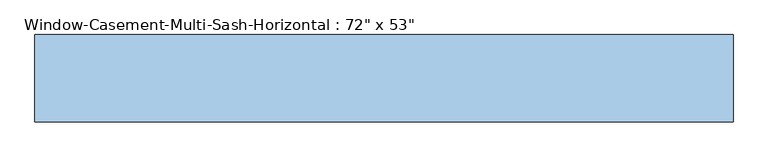
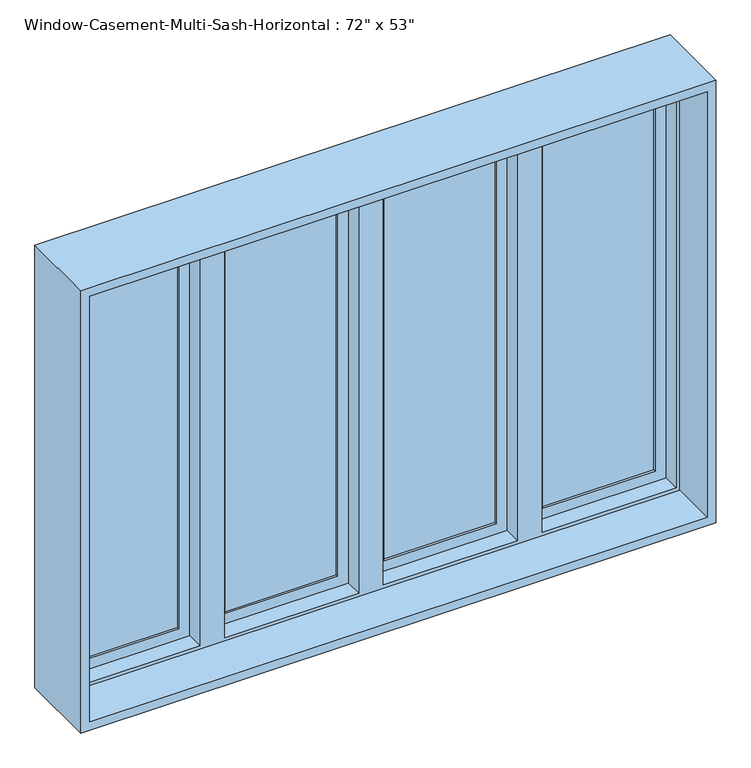
"""IFC4 building model written with IfcOpenShell, lengths in millimetres: window geometry."""

from ifc_helpers import new_model, si_unit, frame, origin, place, context, project, spatial, polyline, outline, extrude, faceted_brep, source, transform, mapped, element, save


def window_5487fb6d(model_context):
    return source(origin(), model_context, "Body", "SolidModel", [
        extrude(outline(polyline([(2235.2, 482.6), (939.8, 482.6), (939.8, 889.0), (2235.2, 889.0), (2235.2, 482.6)]), holes=[polyline([(2193.3296875, 847.1296875), (981.6703125, 847.1296875), (981.6703125, 524.4703125), (2193.3296875, 524.4703125), (2193.3296875, 847.1296875)])]), frame((0.0, 73.025, 0.0), z_axis=(0.0, 1.0, 0.0), x_axis=(0.0, 0.0, 1.0)), (0.0, 0.0, 1.0), 31.75),
        extrude(outline(polyline([(2235.2, -889.0), (939.8, -889.0), (939.8, -482.6), (2235.2, -482.6), (2235.2, -889.0)]), holes=[polyline([(2193.3296875, -524.4703125), (981.6703125, -524.4703125), (981.6703125, -847.1296875), (2193.3296875, -847.1296875), (2193.3296875, -524.4703125)])]), frame((0.0, 73.025, 0.0), z_axis=(0.0, 1.0, 0.0), x_axis=(0.0, 0.0, 1.0)), (0.0, 0.0, 1.0), 31.75),
        extrude(outline(polyline([(-524.4703125, 98.425), (-524.4703125, 92.075), (-847.1296875, 92.075), (-847.1296875, 98.425), (-524.4703125, 98.425)])), frame((0.0, 0.0, 981.6703125), z_axis=(0.0, 0.0, 1.0), x_axis=(1.0, 0.0, 0.0)), (0.0, 0.0, 1.0), 1211.659375),
        extrude(outline(polyline([(-524.4703125, 85.725), (-524.4703125, 79.375), (-847.1296875, 79.375), (-847.1296875, 85.725), (-524.4703125, 85.725)])), frame((0.0, 0.0, 981.6703125), z_axis=(0.0, 0.0, 1.0), x_axis=(1.0, 0.0, 0.0)), (0.0, 0.0, 1.0), 1211.659375),
        extrude(outline(polyline([(847.1296875, 98.425), (847.1296875, 92.075), (524.4703125, 92.075), (524.4703125, 98.425), (847.1296875, 98.425)])), frame((0.0, 0.0, 981.6703125), z_axis=(0.0, 0.0, 1.0), x_axis=(1.0, 0.0, 0.0)), (0.0, 0.0, 1.0), 1211.659375),
        extrude(outline(polyline([(847.1296875, 85.725), (847.1296875, 79.375), (524.4703125, 79.375), (524.4703125, 85.725), (847.1296875, 85.725)])), frame((0.0, 0.0, 981.6703125), z_axis=(0.0, 0.0, 1.0), x_axis=(1.0, 0.0, 0.0)), (0.0, 0.0, 1.0), 1211.659375),
        extrude(outline(polyline([(-67.2703125, 98.425), (-67.2703125, 92.075), (-389.9296875, 92.075), (-389.9296875, 98.425), (-67.2703125, 98.425)])), frame((0.0, 0.0, 981.6703125), z_axis=(0.0, 0.0, 1.0), x_axis=(1.0, 0.0, 0.0)), (0.0, 0.0, 1.0), 1211.659375),
        extrude(outline(polyline([(-67.2703125, 85.725), (-67.2703125, 79.375), (-389.9296875, 79.375), (-389.9296875, 85.725), (-67.2703125, 85.725)])), frame((0.0, 0.0, 981.6703125), z_axis=(0.0, 0.0, 1.0), x_axis=(1.0, 0.0, 0.0)), (0.0, 0.0, 1.0), 1211.659375),
        extrude(outline(polyline([(389.9296875, 98.425), (389.9296875, 92.075), (67.2703125, 92.075), (67.2703125, 98.425), (389.9296875, 98.425)])), frame((0.0, 0.0, 981.6703125), z_axis=(0.0, 0.0, 1.0), x_axis=(1.0, 0.0, 0.0)), (0.0, 0.0, 1.0), 1211.659375),
        extrude(outline(polyline([(389.9296875, 85.725), (389.9296875, 79.375), (67.2703125, 79.375), (67.2703125, 85.725), (389.9296875, 85.725)])), frame((0.0, 0.0, 981.6703125), z_axis=(0.0, 0.0, 1.0), x_axis=(1.0, 0.0, 0.0)), (0.0, 0.0, 1.0), 1211.659375),
        faceted_brep([(-482.6, 73.025, 2235.2), (-889.0, 73.025, 2235.2), (-889.0, 114.3, 2235.2), (889.0, 114.3, 2235.2), (889.0, 73.025, 2235.2), (482.6, 73.025, 2235.2), (482.6, 111.125, 2235.2), (431.8, 111.125, 2235.2), (431.8, 73.025, 2235.2), (25.4, 73.025, 2235.2), (25.4, 111.125, 2235.2), (-25.4, 111.125, 2235.2), (-25.4, 73.025, 2235.2), (-431.8, 73.025, 2235.2), (-431.8, 111.125, 2235.2), (-482.6, 111.125, 2235.2), (-878.8796875, 22.225, 2225.0796875), (-878.8796875, 73.025, 2225.0796875), (-492.7203125, 73.025, 2225.0796875), (-492.7203125, 22.225, 2225.0796875), (878.8796875, 73.025, 2225.0796875), (878.8796875, 22.225, 2225.0796875), (492.7203125, 22.225, 2225.0796875), (492.7203125, 73.025, 2225.0796875), (-421.6796875, 73.025, 2225.0796875), (-35.5203125, 73.025, 2225.0796875), (-35.5203125, 22.225, 2225.0796875), (-421.6796875, 22.225, 2225.0796875), (35.5203125, 73.025, 2225.0796875), (421.6796875, 73.025, 2225.0796875), (421.6796875, 22.225, 2225.0796875), (35.5203125, 22.225, 2225.0796875), (-889.0, -114.3, 2235.2), (-889.0, 22.225, 2235.2), (889.0, 22.225, 2235.2), (889.0, -114.3, 2235.2), (-914.4, 114.3, 2260.6), (-914.4, -114.3, 2260.6), (914.4, -114.3, 2260.6), (914.4, 114.3, 2260.6), (889.0, 114.3, 939.8), (889.0, 73.025, 939.8), (878.8796875, 73.025, 949.9203125), (878.8796875, 22.225, 949.9203125), (889.0, 22.225, 939.8), (889.0, -114.3, 939.8), (914.4, -114.3, 914.4), (914.4, 114.3, 914.4), (482.6, 73.025, 939.8), (-889.0, 114.3, 939.8), (-889.0, 73.025, 939.8), (-482.6, 73.025, 939.8), (-482.6, 111.125, 939.8), (-431.8, 111.125, 939.8), (-431.8, 73.025, 939.8), (-25.4, 73.025, 939.8), (-25.4, 111.125, 939.8), (25.4, 111.125, 939.8), (25.4, 73.025, 939.8), (431.8, 73.025, 939.8), (431.8, 111.125, 939.8), (482.6, 111.125, 939.8), (492.7203125, 73.025, 949.9203125), (492.7203125, 22.225, 949.9203125), (-878.8796875, 73.025, 949.9203125), (-878.8796875, 22.225, 949.9203125), (-492.7203125, 22.225, 949.9203125), (-492.7203125, 73.025, 949.9203125), (-35.5203125, 73.025, 949.9203125), (-421.6796875, 73.025, 949.9203125), (-421.6796875, 22.225, 949.9203125), (-35.5203125, 22.225, 949.9203125), (421.6796875, 73.025, 949.9203125), (35.5203125, 73.025, 949.9203125), (35.5203125, 22.225, 949.9203125), (421.6796875, 22.225, 949.9203125), (-889.0, 22.225, 939.8), (-889.0, -114.3, 939.8), (-914.4, -114.3, 914.4), (-914.4, 114.3, 914.4)], [[[0, 1, 2, 3, 4, 5, 6, 7, 8, 9, 10, 11, 12, 13, 14, 15]], [[16, 17, 18, 19]], [[20, 21, 22, 23]], [[24, 25, 26, 27]], [[28, 29, 30, 31]], [[32, 33, 34, 35]], [[36, 37, 38, 39]], [[4, 3, 40, 41]], [[21, 20, 42, 43]], [[35, 34, 44, 45]], [[39, 38, 46, 47]], [[48, 41, 40, 49, 50, 51, 52, 53, 54, 55, 56, 57, 58, 59, 60, 61]], [[43, 42, 62, 63]], [[64, 65, 66, 67]], [[68, 69, 70, 71]], [[72, 73, 74, 75]], [[45, 44, 76, 77]], [[47, 46, 78, 79]], [[2, 1, 50, 49]], [[4, 41, 48, 5], [20, 23, 62, 42]], [[50, 1, 0, 51], [64, 67, 18, 17]], [[12, 55, 54, 13], [69, 68, 25, 24]], [[8, 59, 58, 9], [73, 72, 29, 28]], [[17, 16, 65, 64]], [[44, 34, 33, 76], [16, 19, 66, 65], [27, 26, 71, 70], [31, 30, 75, 74], [21, 43, 63, 22]], [[33, 32, 77, 76]], [[38, 37, 78, 46], [32, 35, 45, 77]], [[37, 36, 79, 78]], [[36, 39, 47, 79], [3, 2, 49, 40]], [[18, 67, 66, 19]], [[69, 24, 27, 70]], [[53, 14, 13, 54]], [[14, 53, 52, 15]], [[15, 52, 51, 0]], [[25, 68, 71, 26]], [[73, 28, 31, 74]], [[57, 10, 9, 58]], [[10, 57, 56, 11]], [[11, 56, 55, 12]], [[6, 61, 60, 7]], [[7, 60, 59, 8]], [[29, 72, 75, 30]], [[62, 23, 22, 63]], [[61, 6, 5, 48]]]),
        extrude(outline(polyline([(2235.2, 25.4), (939.8, 25.4), (939.8, 431.8), (2235.2, 431.8), (2235.2, 25.4)]), holes=[polyline([(2193.3296875, 389.9296875), (981.6703125, 389.9296875), (981.6703125, 67.2703125), (2193.3296875, 67.2703125), (2193.3296875, 389.9296875)])]), frame((0.0, 73.025, 0.0), z_axis=(0.0, 1.0, 0.0), x_axis=(0.0, 0.0, 1.0)), (0.0, 0.0, 1.0), 31.75),
        extrude(outline(polyline([(2235.2, -431.8), (939.8, -431.8), (939.8, -25.4), (2235.2, -25.4), (2235.2, -431.8)]), holes=[polyline([(2193.3296875, -67.2703125), (981.6703125, -67.2703125), (981.6703125, -389.9296875), (2193.3296875, -389.9296875), (2193.3296875, -67.2703125)])]), frame((0.0, 73.025, 0.0), z_axis=(0.0, 1.0, 0.0), x_axis=(0.0, 0.0, 1.0)), (0.0, 0.0, 1.0), 31.75),
    ])


if __name__ == "__main__":
    model = new_model("IFC4")
    model_context = context("Model", 3, world=origin())
    ifc_project = project(units=[si_unit("LENGTHUNIT", "METRE", prefix="MILLI")], contexts=[model_context])
    site = spatial("IfcSite", under=ifc_project)
    building = spatial("IfcBuilding", under=site)
    placement = place(None, origin())
    window_shape = window_5487fb6d(model_context)
    element("IfcWindow", 1, ObjectType="Window-Casement-Multi-Sash-Horizontal : 72\" x 53\"", at=placement, inside=building, context=model_context, shape_type="MappedRepresentation", body=[
        mapped(window_shape, transform((0.0, 0.0, 0.0), x_axis=(1.0, 0.0, 0.0), y_axis=(0.0, 1.0, 0.0), z_axis=(0.0, 0.0, 1.0))),
    ])
    save(model, "model.ifc")

# Revit data of these elements
# Type "Window-Casement-Multi-Sash-Horizontal : 72\" x 53\""
#   Type Mark = "18"
#   Fire Rating = "0.5h"
#   Assembly Code = "B2020100"
#   Analytic Construction = "Double glazing - domestic"
#   Window Inset [instance default] = 0' - 0 5/8"
#   Wall Thickness [instance default] = 0' - 6"
#   Visual Light Transmittance = 0.81
#   Thermal Resistance (R) = 1.8146 (h·ft²·°F)/BTU
#   Solar Heat Gain Coefficient = 0.76
#   Rough Width = 6' - 0 1/2"
#   Rough Height = 4' - 5 1/2"
#   Open Window Width = 1' - 6"
#   Heat Transfer Coefficient (U) = 0.5511 BTU/(h·ft²·°F)
#   Height = 4' - 5"
#   Frame Gap 3 [instance default] = 0' - 1 83/128"
#   Frame Gap 2 [instance default] = 0' - 0 5/8"
#   Frame Gap 1 = 0' - 1 51/128"
#   Default Sill Height = 3' - 0"
#   Width = 6' - 0"
#   Frame Material = Metal - Aluminum
#   Glass Panel Material = Glass
#   Wall Closure = (empty or 0)
# Element 1 (IfcWindow, "Window-Casement-Multi-Sash-Horizontal : 72\" x 53\"")
#   Wall Thickness = 0' - 9"
#   Materials on its faces: "Metal - Aluminum", "Glass"
# Materials
#   "Metal - Aluminum": class "Metal", colour RGB 247 247 247, transparency 0
#   "Glass": class "Glass", colour RGB 0 128 192, transparency 0.75, Description = "Soda Lime Glass", Cost = 0
